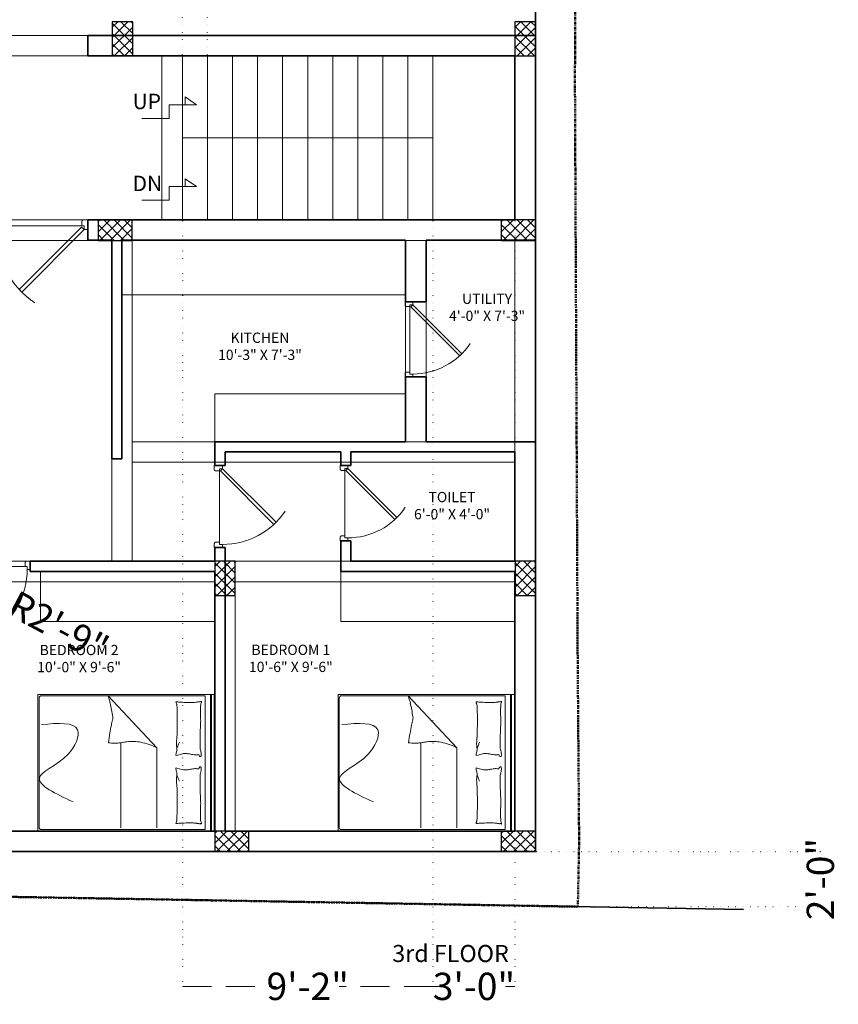
# Model space of a CAD drawing. Units: inches. Extents: x -16911 to -9621, y -48626 to -46270.
# Tile 18 of 20: x -11365 to -11006, y -47012 to -46579. Entities that reach past the tile are written whole.
import ezdxf

# ---------------------------------------------------------------- set-up
doc = ezdxf.new("R2010")
doc.units = ezdxf.units.IN
for name, pattern in [('DASHDOT', [1, 0.5, -0.25, 0, -0.25]), ('DASHED', [19.05, 12.7, -6.35]), ('DOT2', [3.175, 0, -3.175])]:
    doc.linetypes.add(name, pattern=pattern)
for name, color, linetype, lineweight in [('A-ANNO-DIMS', 2, 'Continuous', 13), ('A-ANNO-SYMB', 3, 'Continuous', 13), ('A-ANNO-TEXT', 7, 'Continuous', 18), ('A-AREA-IDEN', 3, 'Continuous', 18), ('A-DOOR', 4, 'Continuous', 18), ('A-FLOR-STRS', 3, 'Continuous', 18), ('A-FURN', 8, 'Continuous', 13), ('A-WALL', 7, 'Continuous', 35), ('C-PROP', 6, 'DASHDOT', 50), ('column', 12, 'Continuous', 30), ('DOOR', 143, 'Continuous', 9), ('EXT BEAM', 132, 'Continuous', 13), ('furniture', 35, 'Continuous', 15), ('S-BEAM', 132, 'Continuous', 25), ('S-COLS', 1, 'Continuous', 30), ('STAIRCASE', 137, 'Continuous', 5)]:
    doc.layers.add(name, color=color, linetype=linetype, lineweight=lineweight)
doc.styles.get("Standard").update_dxf_attribs({"font": 'swissel.ttf'})
doc.styles.add('style9', font='swisscl.ttf', dxfattribs={"height": 12})
doc.dimstyles.new('Dim9', dxfattribs={"dimtxt": 10, "dimasz": 0.199219, "dimexe": 1, "dimexo": 0.5, "dimgap": 1, "dimtad": 0, "dimdec": 1, "dimzin": 0, "dimdsep": 46, "dimlunit": 4, "dimtxsty": 'style9', "dimblk": 'ARCHTICK', "dimcen": 0.09, "dimclrd": 256, "dimclrt": 256, "dimadec": 0, "dimazin": 0, "dimtfac": 1, "dimtdec": 1, "dimtix": 1, "dimtofl": 0, "dimtmove": 1, "dimatfit": 3, "dimfxl": 9, "dimtolj": 1, "dimtzin": 0, "dimlwd": -1, "dimarcsym": 0})

# ---------------------------------------------------------------- blocks, each defined once
blk = doc.blocks.new('hjuyuiuyk')
at = {"layer": 'furniture'}
for p, q in [((-19327.49, -39738.98), (-19327.49, -39737.31)), ((-19327.49, -39737.31), (-19267.49, -39737.31, 0)), ((-19327.49, -39746.54), (-19327.49, -39737.31)), ((-19267.49, -39738.5), (-19327.49, -39738.5, 0)), ((-19327.49, -39738.5, 0), (-19327.49, -39814.72, 0)), ((-19327.49, -39738.5), (-19327.49, -39814.72)), ((-19267.49, -39738.5, 0), (-19327.49, -39738.5)), ((-19267.49, -39738.98, 0), (-19327.49, -39738.98)), ((-19267.49, -39737.31, 0), (-19267.49, -39738.98, 0)), ((-19267.49, -39746.54, 0), (-19267.49, -39737.31, 0)), ((-19267.49, -39814.72), (-19267.49, -39738.5)), ((-19267.49, -39814.72, 0), (-19267.49, -39738.5, 0)), ((-19268.1, -39741.33), (-19326.9, -39741.33)), ((-19326.9, -39741.33), (-19326.9, -39813.21)), ((-19268.1, -39813.21), (-19268.1, -39741.33)), ((-19300.88, -39753.22, 0), (-19301.49, -39750.81, 0)), ((-19294.97, -39753.22, 0), (-19294.37, -39750.81, 0)), ((-19300.67, -39754.09, 0), (-19300.88, -39753.22, 0)), ((-19295.19, -39754.09, 0), (-19294.97, -39753.22, 0)), ((-19304.07, -39762.52), (-19326.9, -39783.91)), ((-19304.07, -39762.52), (-19268.82, -39762.52)), ((-19268.82, -39778.34), (-19306.29, -39778.34)), ((-19326.9, -39813.21), (-19326.9, -39783.91)), ((-19327.49, -39814.72, 0), (-19267.49, -39814.72)), ((-19327.49, -39814.72), (-19267.49, -39814.72, 0)), ((-19269.1, -39814.21), (-19325.9, -39814.21)), ((-19325.9, -39814.21), (-19269.1, -39814.21))]:
    blk.add_line(p, q, dxfattribs=at)
for centre, radius, start, end in [((-19324.36, -39743.07, 0), 0.0997, 111.7883, 160.436), ((-19324.39, -39743.06, 0), 0.0676, 160.436, 281.8931), ((-19324.12, -39743.66, 0), 0.732, 94.3025, 111.7883), ((-19324.35, -39743.25, 0), 0.125, 21.9904, 101.8931), ((-19323.34, -39743.89, 0), 0.956, 158.579, 188.1335), ((-19324.65, -39743.37, 0), 0.455, 338.579, 21.9904), ((-19324.11, -39743.77, 0), 0.842, 59.3487, 94.3025), ((-19322.88, -39741.69, 0), 1.57, 239.3487, 264.7408), ((-19319.6, -39692.5, 0), 50.87, 266.1399, 268.6002), ((-19319.84, -39713.09, 0), 30.28, 268.0921, 271.2808), ((-19320.24, -39695.07, 0), 48.31, 271.2808, 273.4034), ((-19316.15, -39763.89, 0), 20.63, 90.1553, 93.4034), ((-19316.09, -39783.15, 0), 39.89, 86.9902, 90.1553), ((-19305.86, -39588.51, 0), 155.02, 266.9902, 268.5957), ((-19305.42, -39570.46, 0), 173.07, 268.5957, 270), ((-19305.42, -39718.38, 0), 25.15, 270, 273.6841), ((-19304.03, -39739.9, 0), 3.58, 273.6841, 287.1951), ((-19300.46, -39751.46, 0), 8.51, 98.4372, 107.1951), ((-19301.02, -39747.69, 0), 4.7, 90, 98.4372), ((-19301.12, -39743.14, 0), 0.997, 274.4002, 333.4195), ((-19301.02, -39745.63, 0), 2.64, 78.7276, 90), ((-19300.58, -39743.42, 0), 0.383, 333.4195, 78.7276), ((-19295.28, -39743.42, 0), 0.383, 101.2724, 206.5805), ((-19294.73, -39743.14, 0), 0.997, 206.5805, 265.5998), ((-19294.84, -39745.63, 0), 2.64, 90, 101.2724), ((-19294.84, -39747.69, 0), 4.7, 81.5628, 90), ((-19295.39, -39751.46, 0), 8.51, 72.8049, 81.5628), ((-19291.82, -39739.9, 0), 3.58, 252.8049, 266.3159), ((-19290.43, -39718.38, 0), 25.15, 266.3159, 270), ((-19290.43, -39570.46, 0), 173.07, 270, 271.4043), ((-19289.99, -39588.51, 0), 155.02, 271.4043, 273.0098), ((-19279.76, -39783.15, 0), 39.89, 89.8447, 93.0098), ((-19279.7, -39763.89, 0), 20.63, 86.5966, 89.8447), ((-19275.61, -39695.07, 0), 48.31, 266.5966, 268.7192), ((-19276.02, -39713.09, 0), 30.28, 268.7192, 271.9079), ((-19276.73, -39645.13, 0), 98.25, 271.0069, 272.7772), ((-19272.12, -39741.69, 0), 1.57, 275.2592, 300.6513), ((-19270.89, -39743.77, 0), 0.842, 85.6975, 120.6513), ((-19270.88, -39743.66, 0), 0.732, 68.2117, 85.6975), ((-19270.35, -39743.37, 0), 0.455, 158.0096, 201.421), ((-19270.65, -39743.25, 0), 0.125, 78.1069, 158.0096), ((-19271.66, -39743.89, 0), 0.956, 351.8665, 21.421), ((-19270.61, -39743.06, 0), 0.0676, 258.1069, 19.564), ((-19270.64, -39743.07, 0), 0.0997, 19.564, 68.2117), ((-19317.18, -39743.01, 0), 7.17, 188.1335, 192.1095), ((-19329.85, -39745.73, 0), 5.78, 7.6809, 12.1095), ((-19350.51, -39748.51, 0), 26.62, 3.3687, 7.6809), ((-19343.69, -39748.11, 0), 19.79, 358.3669, 3.3687), ((-19292.22, -39749.75, 0), 9.25, 167.8016, 171.9949), ((-19326.4, -39742.36, 0), 25.72, 347.8016, 350.3156), ((-19315.3, -39745.68, 0), 14.34, 360, 6.2324), ((-19306.91, -39745.68, 0), 5.95, 350.3156, 360), ((-19280.55, -39745.68, 0), 14.34, 173.7676, 180), ((-19288.94, -39745.68, 0), 5.95, 180, 189.6844), ((-19269.45, -39742.36, 0), 25.72, 189.6844, 192.1984), ((-19303.63, -39749.75, 0), 9.25, 8.0051, 12.1984), ((-19251.31, -39748.11, 0), 19.79, 176.6313, 181.6331), ((-19244.49, -39748.51, 0), 26.62, 172.3191, 176.6313), ((-19265.15, -39745.73, 0), 5.78, 167.8905, 172.3191), ((-19277.82, -39743.01, 0), 7.17, 347.8905, 351.8665), ((-19720.99, -39728.47, 0), 397.61, 356.4951, 356.945), ((-19363.7, -39747.54, 0), 39.81, 356.945, 358.3669), ((-19299.57, -39750.33, 0), 1.97, 177.3351, 194.0452), ((-19282.35, -39751.13, 0), 19.21, 171.9949, 177.3351), ((-19313.5, -39751.13, 0), 19.21, 2.6649, 8.0051), ((-19296.28, -39750.33, 0), 1.97, 345.9548, 2.6649), ((-19231.3, -39747.54, 0), 39.81, 181.6331, 183.055), ((-18874.01, -39728.47, 0), 397.61, 183.055, 183.5049), ((-19323.69, -39753.93, 0), 0.564, 170.0016, 196.6978), ((-19333.47, -39752.21, 0), 9.37, 350.0016, 356.4951), ((-19324.19, -39754.08, 0), 0.0385, 196.6978, 277.1204), ((-19324.51, -39751.59, 0), 2.55, 277.1204, 286.2212), ((-19324.42, -39751.9, 0), 2.23, 286.2212, 297.4439), ((-19322.81, -39754.99, 0), 1.25, 102.448, 117.4439), ((-19322.32, -39757.22, 0), 3.54, 93.574, 102.448), ((-19318.44, -39837.61, 0), 84.03, 90.9755, 92.7955), ((-19315.55, -39952.16, 0), 198.61, 89.4461, 91.2473), ((-19314.9, -39885.06, 0), 131.51, 87.2326, 89.4461), ((-19310.57, -39795.48, 0), 41.81, 85.4012, 87.2326), ((-19304.32, -39717.78, 0), 36.14, 265.4012, 267.3712), ((-19297.32, -39733.09, 0), 21.54, 244.6889, 246.5156), ((-19305.66, -39747.05, 0), 6.83, 267.3712, 281.4827), ((-19297.32, -39733.09, 0), 21.54, 246.5156, 248.3423), ((-19297.32, -39733.09, 0), 21.54, 248.3423, 250.572), ((-19297.32, -39733.09, 0), 21.54, 250.572, 252.8018), ((-19303.46, -39757.91, 0), 4.25, 83.5659, 101.4827), ((-19303.37, -39757.16, 0), 3.49, 72.6136, 83.5659), ((-19300.33, -39747.43, 0), 6.7, 252.6136, 260.5159), ((-19300.13, -39746.25, 0), 7.9, 260.5159, 265.9171), ((-19300.69, -39754.1, 0), 0.0267, 265.9171, 14.0449), ((-19295.16, -39754.1, 0), 0.0267, 165.9551, 274.0829), ((-19295.72, -39746.25, 0), 7.9, 274.0829, 279.4841), ((-19295.52, -39747.43, 0), 6.7, 279.4841, 287.3864), ((-19292.48, -39757.16, 0), 3.49, 96.4341, 107.3864), ((-19292.39, -39757.91, 0), 4.25, 78.5173, 96.4341), ((-19298.54, -39733.09, 0), 21.54, 287.1982, 289.428), ((-19290.19, -39747.05, 0), 6.83, 258.5173, 272.6288), ((-19298.54, -39733.09, 0), 21.54, 289.428, 291.6577), ((-19298.54, -39733.09, 0), 21.54, 291.6577, 293.4844), ((-19298.54, -39733.09, 0), 21.54, 293.4844, 295.3111), ((-19291.53, -39717.78, 0), 36.14, 272.6288, 274.5988), ((-19285.28, -39795.48, 0), 41.81, 92.7674, 94.5988), ((-19280.95, -39885.06, 0), 131.51, 90.5539, 92.7674), ((-19280.3, -39952.16, 0), 198.61, 88.7527, 90.5539), ((-19277.1, -39805.01, 0), 51.42, 86.426, 88.7527), ((-19274.68, -39799.75, 0), 46.07, 86.5575, 89.0171), ((-19272.19, -39754.99, 0), 1.25, 62.5561, 77.552), ((-19270.58, -39751.9, 0), 2.23, 242.5561, 253.7788), ((-19270.49, -39751.59, 0), 2.55, 253.7788, 262.8796), ((-19261.53, -39752.21, 0), 9.37, 183.5049, 189.9984), ((-19270.81, -39754.08, 0), 0.0385, 262.8796, 343.3022), ((-19271.31, -39753.93, 0), 0.564, 343.3022, 9.9984), ((-19279.47, -39774.89), 27.53, 153.3084, 168.7423), ((-19287.94, -39773.2), 18.89, 168.7423, 187.3994), ((-19242.78, -39767.34), 64.43, 187.3994, 189.2719), ((-19333.07, -39782.08), 27.05, 6.3817, 9.2719), ((-19287.64, -39956.87), 177.57, 99.7243, 101.7196), ((-19317.24, -39783.9), 2.09, 82.2696, 100.7276), ((-19317.9, -39788.76), 6.99, 76.8096, 82.2696), ((-19295.64, -39693.77), 90.57, 256.8096, 258.3259), ((-19295.11, -39691.23), 93.17, 258.3259, 260.505), ((-19336.71, -39780.62), 30.63, 354.1141, 359.2313), ((-19321.79, -39780.82), 15.7, 359.2313, 6.3817), ((-19306.77, -39846.83), 66.07, 105.9352, 107.7364), ((-19318.41, -39806.06), 23.67, 102.9255, 105.9352), ((-19288.03, -39648.9), 136.08, 260.505, 262.308), ((-19325.9, -39813.21), 1, 180, 270), ((-19269.1, -39813.21), 1, 270, 0)]:
    blk.add_arc(centre, radius, start, end, dxfattribs=at)
blk.add_open_spline([(-19280.24, -39799.21), (-19283.87, -39806.94), (-19290.73, -39821.55), (-19298.08, -39801.09), (-19315.85, -39793.47), (-19314.86, -39805.92), (-19314.29, -39813.13)], degree=3, knots=[0, 0, 0, 0, 18.167809, 34.338432, 45.972904, 61.997799, 61.997799, 61.997799, 61.997799], dxfattribs=at)
blk = doc.blocks.new('A$C1C9D3E54')
at = {"layer": 'DOOR'}
blk.add_line((18676.53, 5780.72), (18710.53, 5780.72), dxfattribs=at)
blk.add_lwpolyline([(18685.01, 5806.62), (18710.47, 5781.16), (18711.53, 5782.22), (18686.07, 5807.68), (18685.01, 5806.62)], dxfattribs=at)
blk.add_lwpolyline([(18674.03, 5778.22), (18676.03, 5778.22), (18674.03, 5778.22), (18674.03, 5782.22), (18675.53, 5782.22), (18675.53, 5780.72), (18676.53, 5780.72), (18676.53, 5778.72), (18676.41, 5778.72), (18676.41, 5778.6, -0.414214), (18676.16, 5778.35), (18676.03, 5778.35), (18676.03, 5778.22)], format="xyb", dxfattribs=at)
blk.add_lwpolyline([(18713.03, 5782.22), (18711.53, 5782.22), (18711.53, 5780.72), (18710.53, 5780.72), (18710.53, 5778.72), (18710.66, 5778.72), (18710.66, 5778.6, 0.414214), (18710.91, 5778.35), (18711.03, 5778.35), (18711.03, 5778.22), (18713.03, 5778.22), (18711.03, 5778.22), (18713.03, 5778.22), (18713.03, 5782.22)], format="xyb", close=True, dxfattribs=at)
blk.add_arc((18711.53, 5782.22), 36, 124.0336, 180, dxfattribs=at)
blk = doc.blocks.new('THYHYTJ')
at = {"layer": 'STAIRCASE', "ltscale": 10}
for p, q in [((-7981.18, -46346.18), (-7984.62, -46351.1)), ((-7981.18, -46358.18), (-7981.18, -46346.18)), ((-7984.62, -46351.1), (-7981.18, -46351.1)), ((-7975.18, -46358.18), (-7981.18, -46358.18)), ((-7975.18, -46370.18), (-7975.18, -46358.18))]:
    blk.add_line(p, q, dxfattribs=at)
blk = doc.blocks.new('COLUMNS')
at = {"layer": 'column'}
h = blk.add_hatch(dxfattribs=at)
h.set_pattern_fill('ANSI37', color=256, angle=-720)
h.set_pattern_definition([(45, (21840.2088, -104675.1704), (-2.24506403, 2.24506403), []), (135, (21840.2088, -104675.1704), (-2.24506403, -2.24506403), [])])
h.paths.add_polyline_path([(-11924.72, -46595.36), (-11915.72, -46595.36), (-11915.72, -46580.36), (-11924.72, -46580.36)])
h = blk.add_hatch(dxfattribs=at)
h.set_pattern_fill('ANSI37', color=256, angle=-900)
h.set_pattern_definition([(225, (-45503.8578, 11499.4594), (2.24506403, -2.24506403), []), (315, (-45503.8578, 11499.4594), (2.24506403, 2.24506403), [])])
h.paths.add_polyline_path([(-11738.92, -46580.36), (-11747.92, -46580.36), (-11747.92, -46595.36), (-11738.92, -46595.36)])
h = blk.add_hatch(dxfattribs=at)
h.set_pattern_fill('ANSI37', color=256, angle=-810)
h.set_pattern_definition([(315, (-70010.7892, -80432.2886), (2.24506403, 2.24506403), []), (45, (-70010.7892, -80432.2886), (-2.24506403, 2.24506403), [])])
h.paths.add_polyline_path([(-11930.97, -46667.36), (-11930.97, -46676.36), (-11915.97, -46676.36), (-11915.97, -46667.36)])
h = blk.add_hatch(dxfattribs=at)
h.set_pattern_fill('ANSI37', color=256, angle=-810)
h.set_pattern_definition([(315, (-69833.7395, -80432.2886), (2.24506403, 2.24506403), []), (45, (-69833.7395, -80432.2886), (-2.24506403, 2.24506403), [])])
h.paths.add_polyline_path([(-11753.92, -46667.36), (-11753.92, -46676.36), (-11738.92, -46676.36), (-11738.92, -46667.36)])
h = blk.add_hatch(dxfattribs=at)
h.set_pattern_fill('ANSI37', color=256, angle=-720)
h.set_pattern_definition([(45, (21885.2088, -104912.1242), (-2.24506403, 2.24506403), []), (135, (21885.2088, -104912.1242), (-2.24506403, -2.24506403), [])])
h.paths.add_polyline_path([(-11879.72, -46832.31), (-11870.72, -46832.31), (-11870.72, -46817.31), (-11879.72, -46817.31)])
h = blk.add_hatch(dxfattribs=at)
h.set_pattern_fill('ANSI37', color=256, angle=-720)
h.set_pattern_definition([(45, (22017.1023, -104912.1242), (-2.24506403, 2.24506403), []), (135, (22017.1023, -104912.1242), (-2.24506403, -2.24506403), [])])
h.paths.add_polyline_path([(-11747.83, -46832.31), (-11738.83, -46832.31), (-11738.83, -46817.31), (-11747.83, -46817.31)])
h = blk.add_hatch(dxfattribs=at)
h.set_pattern_fill('ANSI37', color=256, angle=-810)
h.set_pattern_definition([(315, (-69959.5392, -80700.7425), (2.24506403, 2.24506403), []), (45, (-69959.5392, -80700.7425), (-2.24506403, 2.24506403), [])])
h.paths.add_polyline_path([(-11879.72, -46935.81), (-11879.72, -46944.81), (-11864.72, -46944.81), (-11864.72, -46935.81)])
h = blk.add_hatch(dxfattribs=at)
h.set_pattern_fill('ANSI37', color=256, angle=-810)
h.set_pattern_definition([(315, (-69833.7395, -80700.7425), (2.24506403, 2.24506403), []), (45, (-69833.7395, -80700.7425), (-2.24506403, 2.24506403), [])])
h.paths.add_polyline_path([(-11753.92, -46935.81), (-11753.92, -46944.81), (-11738.92, -46944.81), (-11738.92, -46935.81)])
at = {"layer": 'column', "ltscale": 0.05}
for points in [[(-11915.72, -46580.36), (-11924.72, -46580.36), (-11924.72, -46595.36), (-11915.72, -46595.36)], [(-11747.92, -46595.36), (-11738.92, -46595.36), (-11738.92, -46580.36), (-11747.92, -46580.36)], [(-11915.97, -46676.36), (-11915.97, -46667.36), (-11930.97, -46667.36), (-11930.97, -46676.36)], [(-11738.92, -46676.36), (-11738.92, -46667.36), (-11753.92, -46667.36), (-11753.92, -46676.36)], [(-11870.72, -46817.31), (-11879.72, -46817.31), (-11879.72, -46832.31), (-11870.72, -46832.31)], [(-11738.83, -46817.31), (-11747.83, -46817.31), (-11747.83, -46832.31), (-11738.83, -46832.31)], [(-11864.72, -46944.81), (-11864.72, -46935.81), (-11879.72, -46935.81), (-11879.72, -46944.81)], [(-11738.92, -46944.81), (-11738.92, -46935.81), (-11753.92, -46935.81), (-11753.92, -46944.81)]]:
    blk.add_lwpolyline(points, close=True, dxfattribs=at)
blk = doc.blocks.new('3RD ROOF BEAMS')
at = {"layer": 'EXT BEAM'}
for p, q in [((-11461.47, -46586.36), (-11324.72, -46586.36)), ((-11461.47, -46944.81), (-11461.47, -46586.36)), ((-11320.47, -46586.36), (-11138.92, -46586.36)), ((-11138.92, -46944.81), (-11138.92, -46586.36)), ((-11452.47, -46595.36), (-11324.72, -46595.36)), ((-11392.47, -46595.36), (-11392.47, -46667.36)), ((-11383.47, -46595.36), (-11383.47, -46667.36)), ((-11320.47, -46595.36), (-11147.92, -46595.36)), ((-11302.92, -46595.36), (-11302.92, -46667.36)), ((-11293.92, -46595.36), (-11293.92, -46667.36)), ((-11147.92, -46667.36), (-11147.92, -46595.36)), ((-11446.47, -46667.36), (-11335.47, -46667.36)), ((-11320.47, -46667.36), (-11138.92, -46667.36)), ((-11452.47, -46817.31), (-11452.47, -46676.36)), ((-11446.47, -46676.36), (-11335.47, -46676.36)), ((-11324.97, -46676.36), (-11324.97, -46817.31)), ((-11320.47, -46676.36), (-11138.92, -46676.36)), ((-11315.97, -46676.36), (-11315.97, -46817.31)), ((-11195.92, -46676.36), (-11195.92, -46764.81)), ((-11186.92, -46676.36), (-11186.92, -46764.81)), ((-11147.92, -46817.31), (-11147.92, -46676.36)), ((-11147.92, -46764.81), (-11315.97, -46764.81)), ((-11147.92, -46773.81), (-11315.97, -46773.81)), ((-11452.47, -46817.31), (-11147.92, -46817.31)), ((-11452.47, -46826.31), (-11279.72, -46826.31)), ((-11452.47, -46944.81), (-11452.47, -46826.31)), ((-11408.97, -46826.31), (-11408.97, -46935.81)), ((-11399.97, -46826.31), (-11399.97, -46935.81)), ((-11279.72, -46826.31), (-11279.72, -46935.81)), ((-11270.72, -46826.31), (-11147.92, -46826.31)), ((-11270.72, -46826.31), (-11270.72, -46935.81)), ((-11147.92, -46935.81), (-11147.92, -46826.31)), ((-11452.47, -46935.81), (-11279.72, -46935.81)), ((-11270.72, -46935.81), (-11147.92, -46935.81)), ((-11461.47, -46944.81), (-11138.92, -46944.81))]:
    blk.add_line(p, q, dxfattribs=at)
blk = doc.blocks.new('_ArchTick')
at = {"color": 0, "linetype": 'ByBlock', "const_width": 0.15}
blk.add_lwpolyline([(-0.5, -0.5), (0.5, 0.5)], dxfattribs=at)
blk = doc.blocks.new('*D123')
at = {"layer": 'A-ANNO-DIMS', "linetype": 'DASHED', "transparency": 16777216}
for p, q in [((-11293.92, -46329.06), (-11294.12, -46329.06)), ((-11282.92, -46329.06), (-11282.73, -46329.06))]:
    blk.add_line(p, q, dxfattribs=at)
at = {"layer": 'A-ANNO-DIMS', "color": 0, "linetype": 'DOT2', "lineweight": -2, "transparency": 16777216}
for p, q in [((-11293.92, -46594.86), (-11293.92, -46328.06)), ((-11282.92, -46594.86), (-11282.92, -46328.06))]:
    blk.add_line(p, q, dxfattribs=at)
at = {"layer": 'Defpoints', "color": 0, "transparency": 16777216}
for p in [(-11282.92, -46329.06), (-11293.92, -46595.36), (-11282.92, -46595.36)]:
    blk.add_point(p, dxfattribs=at)
at = {"layer": 'A-ANNO-DIMS', "transparency": 16777216, "xscale": 0.19921875, "yscale": 0.19921875, "zscale": 0.19921875}
blk.add_blockref('_ArchTick', (-11293.92, -46329.06), dxfattribs=at)
at = {"layer": 'A-ANNO-DIMS', "transparency": 16777216, "xscale": 0.19921875, "yscale": 0.19921875, "zscale": 0.19921875, "rotation": 180}
blk.add_blockref('_ArchTick', (-11282.92, -46329.06), dxfattribs=at)
at = {"layer": 'A-ANNO-DIMS', "transparency": 16777216, "insert": (-11288.42, -46329.06), "char_height": 12, "attachment_point": 5, "style": 'style9'}
blk.add_mtext('\\A1;0\'-11"', dxfattribs=at)
blk = doc.blocks.new('*D124')
at = {"layer": 'A-ANNO-DIMS', "color": 0, "linetype": 'DOT2', "lineweight": -2, "transparency": 16777216}
for p, q in [((-11293.92, -46667.86), (-11293.92, -47005.04)), ((-11183.92, -46667.86), (-11183.92, -47005.04))]:
    blk.add_line(p, q, dxfattribs=at)
at = {"layer": 'A-ANNO-DIMS', "linetype": 'DASHED', "transparency": 16777216}
for p, q in [((-11293.92, -47004.04), (-11252.75, -47004.04)), ((-11183.92, -47004.04), (-11225.1, -47004.04))]:
    blk.add_line(p, q, dxfattribs=at)
at = {"layer": 'Defpoints', "color": 0, "transparency": 16777216}
for p in [(-11293.92, -46667.36), (-11183.92, -46667.36), (-11183.92, -47004.04)]:
    blk.add_point(p, dxfattribs=at)
at = {"layer": 'A-ANNO-DIMS', "transparency": 16777216, "xscale": 0.19921875, "yscale": 0.19921875, "zscale": 0.19921875, "rotation": 180}
blk.add_blockref('_ArchTick', (-11293.92, -47004.04), dxfattribs=at)
at = {"layer": 'A-ANNO-DIMS', "transparency": 16777216, "xscale": 0.19921875, "yscale": 0.19921875, "zscale": 0.19921875}
blk.add_blockref('_ArchTick', (-11183.92, -47004.04), dxfattribs=at)
at = {"layer": 'A-ANNO-DIMS', "transparency": 16777216, "insert": (-11238.92, -47004.04), "char_height": 12, "attachment_point": 5, "style": 'style9'}
blk.add_mtext('\\A1;9\'-2"', dxfattribs=at)
blk = doc.blocks.new('*D125')
at = {"layer": 'A-ANNO-DIMS', "color": 0, "linetype": 'DOT2', "lineweight": -2, "transparency": 16777216}
for p, q in [((-11183.92, -46667.86), (-11183.92, -47005.04)), ((-11147.92, -46667.86), (-11147.92, -47005.04))]:
    blk.add_line(p, q, dxfattribs=at)
at = {"layer": 'A-ANNO-DIMS', "linetype": 'DASHED', "transparency": 16777216}
for p, q in [((-11183.92, -47004.04), (-11179.73, -47004.04)), ((-11147.92, -47004.04), (-11152.12, -47004.04))]:
    blk.add_line(p, q, dxfattribs=at)
at = {"layer": 'Defpoints', "color": 0, "transparency": 16777216}
for p in [(-11183.92, -46667.36), (-11147.92, -46667.36), (-11147.92, -47004.04)]:
    blk.add_point(p, dxfattribs=at)
at = {"layer": 'A-ANNO-DIMS', "transparency": 16777216, "xscale": 0.19921875, "yscale": 0.19921875, "zscale": 0.19921875, "rotation": 180}
blk.add_blockref('_ArchTick', (-11183.92, -47004.04), dxfattribs=at)
at = {"layer": 'A-ANNO-DIMS', "transparency": 16777216, "xscale": 0.19921875, "yscale": 0.19921875, "zscale": 0.19921875}
blk.add_blockref('_ArchTick', (-11147.92, -47004.04), dxfattribs=at)
at = {"layer": 'A-ANNO-DIMS', "transparency": 16777216, "insert": (-11165.92, -47004.04), "char_height": 12, "attachment_point": 5, "style": 'style9'}
blk.add_mtext('\\A1;3\'-0"', dxfattribs=at)
blk = doc.blocks.new('*D129')
at = {"layer": 'A-ANNO-DIMS', "color": 0, "linetype": 'DOT2', "lineweight": -2, "transparency": 16777216}
for p, q in [((-11138.42, -46944.81), (-11012.8, -46944.81)), ((-11119.79, -46969.03), (-11012.8, -46969.03))]:
    blk.add_line(p, q, dxfattribs=at)
at = {"layer": 'A-ANNO-DIMS', "linetype": 'DASHED', "transparency": 16777216}
for p, q in [((-11013.8, -46944.81), (-11013.8, -46944.61)), ((-11013.8, -46969.03), (-11013.8, -46969.23))]:
    blk.add_line(p, q, dxfattribs=at)
at = {"layer": 'Defpoints', "color": 0, "transparency": 16777216}
for p in [(-11138.92, -46944.81), (-11013.8, -46944.81), (-11120.29, -46969.03)]:
    blk.add_point(p, dxfattribs=at)
at = {"layer": 'A-ANNO-DIMS', "transparency": 16777216, "xscale": 0.19921875, "yscale": 0.19921875, "zscale": 0.19921875}
for p, rotation in [((-11013.8, -46944.81), 270), ((-11013.8, -46969.03), 90)]:
    blk.add_blockref('_ArchTick', p, dxfattribs=dict(at, rotation=rotation))
at = {"layer": 'A-ANNO-DIMS', "transparency": 16777216, "insert": (-11013.8, -46956.92), "char_height": 12, "attachment_point": 5, "rotation": 90, "style": 'style9'}
blk.add_mtext('\\A1;2\'-0"', dxfattribs=at)
blk = doc.blocks.new('*D137')
at = {"layer": 'A-ANNO-DIMS', "color": 0, "lineweight": -2, "transparency": 16777216}
for p, q in [((-11395.43, -46821), (-11395.25, -46821)), ((-11395.34, -46821.09), (-11395.34, -46820.91))]:
    blk.add_line(p, q, dxfattribs=at)
at = {"layer": 'A-ANNO-DIMS', "linetype": 'DASHED', "transparency": 16777216}
blk.add_line((-11364.07, -46837.61), (-11365.99, -46836.59), dxfattribs=at)
at = {"layer": 'Defpoints', "color": 0, "transparency": 16777216}
for p in [(-11395.34, -46821), (-11365.99, -46836.59)]:
    blk.add_point(p, dxfattribs=at)
at = {"layer": 'A-ANNO-DIMS', "transparency": 16777216, "xscale": 0.19921875, "yscale": 0.19921875, "zscale": 0.19921875, "rotation": 152.0175078160649}
blk.add_blockref('_ArchTick', (-11365.99, -46836.59), dxfattribs=at)
at = {"layer": 'A-ANNO-DIMS', "transparency": 16777216, "insert": (-11348.39, -46845.95), "char_height": 12, "attachment_point": 5, "rotation": 332.0175, "style": 'style9'}
blk.add_mtext('\\A1;R2\'-9"', dxfattribs=at)

msp = doc.modelspace()

# ---------------------------------------------------------------- linework, layer by layer
at = {"layer": 'A-FLOR-STRS', "ltscale": 10}
for p, q in [((-11293.925, -46595.355), (-11293.925, -46667.355)), ((-11282.925, -46595.355), (-11282.925, -46667.355)), ((-11271.925, -46595.355), (-11271.925, -46667.355)), ((-11260.925, -46595.355), (-11260.925, -46667.355)), ((-11249.925, -46595.355), (-11249.925, -46667.355)), ((-11238.925, -46595.355), (-11238.925, -46667.355)), ((-11227.925, -46595.355), (-11227.925, -46667.355)), ((-11216.925, -46595.355), (-11216.925, -46667.355)), ((-11205.925, -46595.355), (-11205.925, -46667.355)), ((-11194.925, -46595.355), (-11194.925, -46667.355)), ((-11183.925, -46595.355), (-11183.925, -46667.355)), ((-11183.925, -46631.355), (-11293.925, -46631.355))]:
    msp.add_line(p, q, dxfattribs=at)
at = {"layer": 'A-FURN', "ltscale": 0.2}
for p, q in [((-11195.925, -46700.355), (-11320.474, -46700.355)), ((-11195.925, -46743.809), (-11279.724, -46743.809)), ((-11279.724, -46764.809), (-11279.724, -46743.809)), ((-11356.224, -46821.809, 0), (-11356.224, -46843.809, 0)), ((-11224.425, -46821.809), (-11224.425, -46843.809)), ((-11279.724, -46843.809), (-11356.224, -46843.809)), ((-11224.425, -46843.809), (-11147.925, -46843.809))]:
    msp.add_line(p, q, dxfattribs=at)
at = {"layer": 'A-WALL'}
for p, q in [((-11138.925, -46386.855), (-11138.925, -46586.355)), ((-11138.925, -46586.355), (-11335.474, -46586.355)), ((-11335.474, -46595.355), (-11335.474, -46586.355)), ((-11138.925, -46586.355), (-11138.925, -46676.355)), ((-11147.925, -46595.355), (-11335.474, -46595.355)), ((-11147.925, -46595.355), (-11147.925, -46667.355)), ((-11147.925, -46667.355), (-11335.474, -46667.355)), ((-11335.474, -46676.355), (-11335.474, -46667.355)), ((-11324.974, -46676.355), (-11335.474, -46676.355)), ((-11324.974, -46676.355), (-11324.974, -46772.355)), ((-11195.925, -46676.355), (-11320.474, -46676.355)), ((-11320.474, -46676.355), (-11320.474, -46772.355)), ((-11195.925, -46676.355), (-11195.925, -46703.355)), ((-11138.925, -46676.355), (-11186.925, -46676.355)), ((-11186.925, -46676.355), (-11186.925, -46703.355)), ((-11138.925, -46676.355), (-11138.925, -46764.809)), ((-11195.925, -46703.355), (-11186.925, -46703.355)), ((-11195.925, -46736.355), (-11195.925, -46764.809)), ((-11195.925, -46736.355), (-11186.925, -46736.355)), ((-11186.925, -46736.355), (-11186.925, -46764.809)), ((-11279.724, -46775.309), (-11279.724, -46764.809)), ((-11279.724, -46764.809), (-11195.925, -46764.809)), ((-11186.925, -46764.809), (-11138.925, -46764.809)), ((-11138.925, -46764.809), (-11138.925, -46944.809)), ((-11275.224, -46775.309), (-11275.224, -46769.309)), ((-11275.224, -46769.309), (-11224.425, -46769.309)), ((-11224.425, -46769.309), (-11224.425, -46775.309)), ((-11219.925, -46769.309), (-11219.925, -46775.309)), ((-11219.925, -46769.309), (-11147.925, -46769.309)), ((-11147.925, -46769.309), (-11147.925, -46817.309)), ((-11320.474, -46772.355), (-11324.974, -46772.355)), ((-11279.724, -46775.309), (-11275.224, -46775.309)), ((-11224.425, -46775.309), (-11219.925, -46775.309)), ((-11224.425, -46808.309), (-11224.425, -46821.809)), ((-11224.425, -46808.309), (-11219.925, -46808.309)), ((-11219.925, -46808.309), (-11219.925, -46817.309)), ((-11279.724, -46817.309), (-11279.724, -46811.309)), ((-11279.724, -46811.309), (-11275.224, -46811.309)), ((-11275.224, -46935.809), (-11275.224, -46811.309)), ((-11360.724, -46817.309), (-11279.724, -46817.309)), ((-11360.724, -46821.809), (-11360.724, -46817.309)), ((-11219.925, -46817.309), (-11147.925, -46817.309)), ((-11360.724, -46821.809), (-11279.724, -46821.809)), ((-11279.724, -46935.809), (-11279.724, -46821.809)), ((-11224.425, -46821.809), (-11147.925, -46821.809)), ((-11147.925, -46821.809), (-11147.925, -46935.809)), ((-11399.974, -46935.809), (-11279.724, -46935.809)), ((-11275.224, -46935.809), (-11147.925, -46935.809)), ((-11408.974, -46944.809), (-11138.925, -46944.809)), ((-11047.547, -46970.292), (-11554.349, -46961.533))]:
    msp.add_line(p, q, dxfattribs=at)
at = {"layer": 'C-PROP'}
msp.add_lwpolyline([(-11480.474, -46962.809), (-11120.293, -46969.035), (-11119.732, -46940.446), (-11120.395, -46855.606), (-11121.561, -46609.511), (-11121.175, -46367.855), (-11480.838, -46362.811), (-11480.3, -46762.955)], close=True, dxfattribs=at)

# ---------------------------------------------------------------- block references
at = {"layer": 'A-ANNO-SYMB', "rotation": 270.0000000000144}
for p in [(35058.429, -54597.957), (35058.429, -54633.957)]:
    msp.add_blockref('THYHYTJ', p, dxfattribs=at)
at = {"layer": 'A-DOOR'}
for p, xscale, yscale, zscale, rotation in [((-31487.969, -40444.653), -1.076923076922859, 1.076923076922859, 1.076923076922859, 180), ((-16085.441, -62537.458), -0.8461538461538624, 0.8461538461538624, 0.8461538461538624, 270), ((-16613.72, -64048.876), -0.9230769230769229, 0.9230769230769229, 0.9230769230769229, 270), ((-16113.941, -62609.412), -0.8461538461538624, 0.8461538461538624, 0.8461538461538624, 270), ((5876.842, -41483.564), 0.9230769230769229, 0.9230769230769229, 0.9230769230769229, 180)]:
    msp.add_blockref('A$C1C9D3E54', p, dxfattribs=dict(at, xscale=xscale, yscale=yscale, zscale=zscale, rotation=rotation))
at = {"layer": 'A-FURN', "rotation": 270}
for p in [(28457.338, -66203.296), (28589.137, -66203.296, 0)]:
    msp.add_blockref('hjuyuiuyk', p, dxfattribs=at)
at = {"layer": 'S-BEAM'}
msp.add_blockref('3RD ROOF BEAMS', (0, 0), dxfattribs=at)
at = {"layer": 'S-COLS'}
msp.add_blockref('COLUMNS', (600, 0), dxfattribs=at)

# ---------------------------------------------------------------- texts
at = {"layer": 'A-ANNO-TEXT'}
for s, p in [('UP', (-11315.824, -46618.742)), ('DN', (-11315.824, -46654.742))]:
    msp.add_text(s, height=6.75, dxfattribs=at).set_placement(p)
at = {"layer": 'A-ANNO-TEXT', "ltscale": 10, "insert": (-11201.781, -46985.845), "char_height": 7.5, "width": 166.78033, "attachment_point": 1, "style": 'style9'}
msp.add_mtext('\\A1;{\\fCentury Gothic|b0|i0|c0|p34;3rd FLOOR}', dxfattribs=at)
at = {"layer": 'A-AREA-IDEN', "ltscale": 10, "char_height": 4.5, "width": 42.823, "attachment_point": 1, "style": 'style9'}
for s, insert in [('\\A1;\\pxqc;{\\fCentury Gothic|b0|i0|c0|p34;UTILITY\\P4\'-0" X 7\'-3"}', (-11181.564, -46699.772)), ('\\A1;\\pxqc;{\\fCentury Gothic|b0|i0|c0|p34;KITCHEN\\P10\'-3" X 7\'-3"}', (-11281.298, -46716.893)), ('\\A1;\\pxqc;{\\fCentury Gothic|b0|i0|c0|p34;TOILET\\P6\'-0" X 4\'-0"}', (-11196.951, -46786.873)), ('\\A1;\\pxqc;{\\fCentury Gothic|b0|i0|c0|p34;BEDROOM 2\\P10\'-0" X 9\'-6"}', (-11360.722, -46854.047)), ('\\A1;\\pxqc;{\\fCentury Gothic|b0|i0|c0|p34;BEDROOM 1\\P10\'-6" X 9\'-6"}', (-11267.728, -46853.971))]:
    msp.add_mtext(s, dxfattribs=dict(at, insert=insert))

# ---------------------------------------------------------------- dimensions: what is measured, and where the dimension line sits
at = {"layer": 'A-ANNO-DIMS'}
for base, p1, p2, picture, middle in [((-11282.925, -46329.061), (-11293.925, -46595.355), (-11282.925, -46595.355), '*D123', (-11288.425, -46329.061)), ((-11183.925, -47004.042), (-11293.925, -46667.355), (-11183.925, -46667.355), '*D124', (-11238.925, -47004.042)), ((-11147.925, -47004.042), (-11183.925, -46667.355), (-11147.925, -46667.355), '*D125', (-11165.925, -47004.042))]:
    dim = msp.add_linear_dim(base=base, p1=p1, p2=p2, dimstyle='Dim9', override={"dimdec": 1, "dimlfac": 1, "dimrnd": 0, "dimzin": 1, "dimdsep": 46, "dimlunit": 4, "dimfrac": 2}, dxfattribs=at)
    dim.commit()
    dim.dimension.update_dxf_attribs({"geometry": picture, "text_midpoint": middle})
dim = msp.add_radius_dim(center=(-11395.34, -46820.998), mpoint=(-11365.994, -46836.59), dimstyle='Dim9', override={"dimdec": 1, "dimlfac": 1, "dimrnd": 0, "dimzin": 1, "dimdsep": 46, "dimlunit": 4, "dimfrac": 2}, dxfattribs=at)
dim.commit()
dim.dimension.update_dxf_attribs({"geometry": '*D137', "text_midpoint": (-11348.386, -46845.945), "dimtype": 164})
dim = msp.add_linear_dim(base=(-11013.797, -46944.809), p1=(-11120.293, -46969.035), p2=(-11138.925, -46944.809), angle=90, dimstyle='Dim9', override={"dimdec": 1, "dimlfac": 1, "dimrnd": 0, "dimzin": 1, "dimdsep": 46, "dimlunit": 4, "dimfrac": 2}, dxfattribs=at)
dim.commit()
dim.dimension.update_dxf_attribs({"geometry": '*D129', "text_midpoint": (-11013.797, -46956.922)})

doc.saveas('drawing.dxf')
